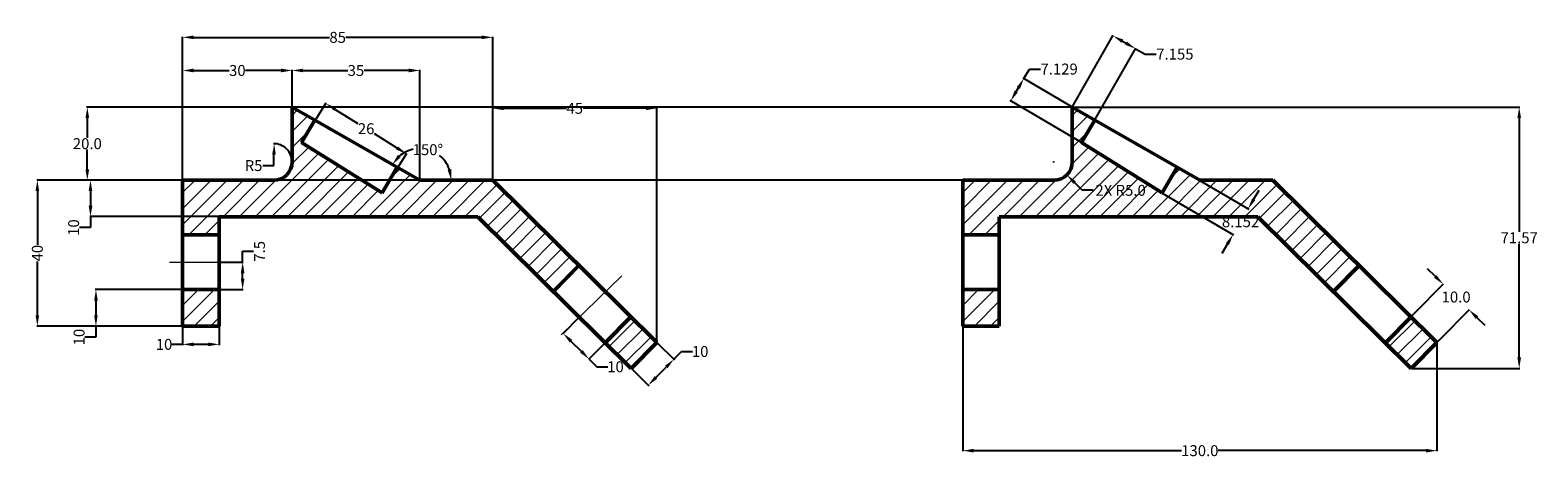
# Model space of a CAD drawing. Units: millimetres. Extents: x 10 to 424, y 8 to 126.
import ezdxf

# ---------------------------------------------------------------- set-up
doc = ezdxf.new("R2010")
doc.units = ezdxf.units.MM
doc.header["$MEASUREMENT"] = 0
doc.linetypes.add('CENTER', pattern=[50.8, 31.75, -6.35, 6.35, -6.35])
for name, color, linetype, lineweight in [('M-CNTR', 4, 'CENTER', 18), ('M-DIMS', 3, 'Continuous', 25), ('M-HATC', 8, 'Continuous', 18), ('M-OUTL', 7, 'Continuous', 50)]:
    doc.layers.add(name, color=color, linetype=linetype, lineweight=lineweight)
doc.styles.get("Standard").update_dxf_attribs({"font": 'arial.ttf'})
doc.dimstyles.get("Standard").update_dxf_attribs({"dimtxt": 3, "dimasz": 3, "dimexe": 0.18, "dimexo": 0.0625, "dimgap": 0.09, "dimtad": 0, "dimtih": 1, "dimtoh": 1, "dimdec": 1, "dimdsep": 46, "dimtxsty": 'Standard', "dimcen": 0.09, "dimadec": 0, "dimazin": 0, "dimtfac": 1, "dimtdec": 1, "dimtofl": 0, "dimtmove": 0, "dimatfit": 3, "dimfxl": 1, "dimtolj": 1, "dimtzin": 0, "dimarcsym": 0})

# ---------------------------------------------------------------- blocks, each defined once
blk = doc.blocks.new('*D1')
at = {"layer": 'Defpoints', "color": 0, "transparency": 16777216}
for p in [(84.8, 94.7), (113.54, 91.62), (106.86, 80.92)]:
    blk.add_point(p, dxfattribs=at)
at = {"layer": 'M-DIMS', "color": 0, "lineweight": -2, "transparency": 16777216}
for p, q in [((84.83, 94.75), (91.58, 105.56)), ((94.03, 103.81), (100.25, 99.93)), ((111, 93.21), (104.78, 97.1)), ((106.89, 80.97), (113.64, 91.77))]:
    blk.add_line(p, q, dxfattribs=at)
at = {"layer": 'M-DIMS', "color": 0, "transparency": 16777216}
for points in [[(94.3, 104.24), (93.77, 103.39), (91.49, 105.4)], [(111.26, 93.63), (110.73, 92.79), (113.54, 91.62)]]:
    blk.add_solid(points, dxfattribs=at)
at = {"layer": 'M-DIMS', "color": 0, "transparency": 16777216, "insert": (102.51, 98.51), "char_height": 3, "attachment_point": 5}
blk.add_mtext('\\A1;26', dxfattribs=at)
blk = doc.blocks.new('*D2')
at = {"layer": 'Defpoints', "color": 0, "transparency": 16777216}
for p in [(137.2, 123.54), (52.2, 84.4), (137.2, 84.4)]:
    blk.add_point(p, dxfattribs=at)
at = {"layer": 'M-DIMS', "color": 0, "lineweight": -2, "transparency": 16777216}
for p, q in [((52.2, 84.46), (52.2, 123.72)), ((55.2, 123.54), (92.44, 123.54)), ((134.2, 123.54), (96.95, 123.54)), ((137.2, 84.46), (137.2, 123.72))]:
    blk.add_line(p, q, dxfattribs=at)
at = {"layer": 'M-DIMS', "color": 0, "transparency": 16777216}
for points in [[(55.2, 124.04), (55.2, 123.04), (52.2, 123.54)], [(134.2, 124.04), (134.2, 123.04), (137.2, 123.54)]]:
    blk.add_solid(points, dxfattribs=at)
at = {"layer": 'M-DIMS', "color": 0, "transparency": 16777216, "insert": (94.7, 123.54), "char_height": 3, "attachment_point": 5}
blk.add_mtext('\\A1;85', dxfattribs=at)
blk = doc.blocks.new('*D3')
at = {"layer": 'Defpoints', "color": 0, "transparency": 16777216}
for p in [(82.2, 114.46), (82.2, 104.4), (52.2, 84.4)]:
    blk.add_point(p, dxfattribs=at)
at = {"layer": 'M-DIMS', "color": 0, "lineweight": -2, "transparency": 16777216}
for p, q in [((52.2, 84.46), (52.2, 114.64)), ((55.2, 114.46), (64.96, 114.46)), ((79.2, 114.46), (69.43, 114.46)), ((82.2, 104.46), (82.2, 114.64))]:
    blk.add_line(p, q, dxfattribs=at)
at = {"layer": 'M-DIMS', "color": 0, "transparency": 16777216}
for points in [[(55.2, 114.96), (55.2, 113.96), (52.2, 114.46)], [(79.2, 114.96), (79.2, 113.96), (82.2, 114.46)]]:
    blk.add_solid(points, dxfattribs=at)
at = {"layer": 'M-DIMS', "color": 0, "transparency": 16777216, "insert": (67.2, 114.46), "char_height": 3, "attachment_point": 5}
blk.add_mtext('\\A1;30', dxfattribs=at)
blk = doc.blocks.new('*D4')
at = {"layer": 'Defpoints', "color": 0, "transparency": 16777216}
for p in [(117.2, 114.46), (82.2, 104.4), (117.2, 84.4)]:
    blk.add_point(p, dxfattribs=at)
at = {"layer": 'M-DIMS', "color": 0, "lineweight": -2, "transparency": 16777216}
for p, q in [((82.2, 104.46), (82.2, 114.64)), ((85.2, 114.46), (97.45, 114.46)), ((114.2, 114.46), (101.94, 114.46)), ((117.2, 84.46), (117.2, 114.64))]:
    blk.add_line(p, q, dxfattribs=at)
at = {"layer": 'M-DIMS', "color": 0, "transparency": 16777216}
for points in [[(85.2, 114.96), (85.2, 113.96), (82.2, 114.46)], [(114.2, 114.96), (114.2, 113.96), (117.2, 114.46)]]:
    blk.add_solid(points, dxfattribs=at)
at = {"layer": 'M-DIMS', "color": 0, "transparency": 16777216, "insert": (99.7, 114.46), "char_height": 3, "attachment_point": 5}
blk.add_mtext('\\A1;35', dxfattribs=at)
blk = doc.blocks.new('*D5')
at = {"layer": 'Defpoints', "color": 0, "transparency": 16777216}
for p in [(77.31, 94.39), (77.2, 89.4)]:
    blk.add_point(p, dxfattribs=at)
at = {"layer": 'M-DIMS', "color": 0, "lineweight": -2, "transparency": 16777216}
for p, q in [((77.17, 88.4), (77.24, 91.4)), ((74.17, 88.4), (77.17, 88.4))]:
    blk.add_line(p, q, dxfattribs=at)
blk.add_arc((77.2, 89.4), 5, 0.7162, 90.7276, dxfattribs=at)
at = {"layer": 'M-DIMS', "color": 0, "transparency": 16777216}
blk.add_solid([(76.74, 91.41), (77.74, 91.38), (77.31, 94.39)], dxfattribs=at)
at = {"layer": 'M-DIMS', "color": 0, "transparency": 16777216, "insert": (71.65, 88.4), "char_height": 3, "attachment_point": 5}
blk.add_mtext('\\A1;R5', dxfattribs=at)
blk = doc.blocks.new('*D6')
at = {"layer": 'Defpoints', "color": 0, "transparency": 16777216}
for p in [(82.2, 104.4), (122.75, 91.04), (117.2, 84.4), (117.2, 84.4), (137.2, 84.4)]:
    blk.add_point(p, dxfattribs=at)
at = {"layer": 'M-DIMS', "color": 0, "lineweight": -2, "transparency": 16777216}
for start, end in [(102.2372, 130.2991), (19.956, 51.1846)]:
    blk.add_arc((117.2, 84.4), 8.66, start, end, dxfattribs=at)
at = {"layer": 'M-DIMS', "color": 0, "transparency": 16777216}
for points in [[(111.98, 90.68), (111.21, 91.32), (109.68, 88.69)], [(125.83, 87.44), (124.84, 87.26), (125.85, 84.4)]]:
    blk.add_solid(points, dxfattribs=at)
at = {"layer": 'M-DIMS', "color": 0, "transparency": 16777216, "insert": (119.42, 92.76), "char_height": 3, "attachment_point": 5}
blk.add_mtext('\\A1;150°', dxfattribs=at)
blk = doc.blocks.new('*D7')
at = {"layer": 'Defpoints', "color": 0, "transparency": 16777216}
for p in [(52.2, 84.4), (26.94, 74.4), (62.2, 74.4)]:
    blk.add_point(p, dxfattribs=at)
at = {"layer": 'M-DIMS', "color": 0, "lineweight": -2, "transparency": 16777216}
for p, q in [((52.13, 84.4), (26.76, 84.4)), ((26.94, 81.4), (26.94, 77.4)), ((26.94, 71.4), (23.94, 71.4)), ((62.13, 74.4), (26.76, 74.4)), ((26.94, 74.4), (26.94, 71.4))]:
    blk.add_line(p, q, dxfattribs=at)
at = {"layer": 'M-DIMS', "color": 0, "transparency": 16777216}
for points in [[(26.44, 81.4), (27.44, 81.4), (26.94, 84.4)], [(26.44, 77.4), (27.44, 77.4), (26.94, 74.4)]]:
    blk.add_solid(points, dxfattribs=at)
at = {"layer": 'M-DIMS', "color": 0, "transparency": 16777216, "insert": (22.32, 71.4), "char_height": 3, "attachment_point": 5, "rotation": 90}
blk.add_mtext('\\A1;10', dxfattribs=at)
blk = doc.blocks.new('*D8')
at = {"layer": 'Defpoints', "color": 0, "transparency": 16777216}
for p in [(52.2, 54.4), (28.43, 44.4), (52.2, 44.4)]:
    blk.add_point(p, dxfattribs=at)
at = {"layer": 'M-DIMS', "color": 0, "lineweight": -2, "transparency": 16777216}
for p, q in [((52.13, 54.4), (28.25, 54.4)), ((28.43, 51.4), (28.43, 47.4)), ((28.43, 41.4), (25.43, 41.4)), ((52.13, 44.4), (28.25, 44.4)), ((28.43, 44.4), (28.43, 41.4))]:
    blk.add_line(p, q, dxfattribs=at)
at = {"layer": 'M-DIMS', "color": 0, "transparency": 16777216}
for points in [[(27.93, 51.4), (28.93, 51.4), (28.43, 54.4)], [(27.93, 47.4), (28.93, 47.4), (28.43, 44.4)]]:
    blk.add_solid(points, dxfattribs=at)
at = {"layer": 'M-DIMS', "color": 0, "transparency": 16777216, "insert": (23.81, 41.4), "char_height": 3, "attachment_point": 5, "rotation": 90}
blk.add_mtext('\\A1;10', dxfattribs=at)
blk = doc.blocks.new('*D9')
at = {"layer": 'Defpoints', "color": 0, "transparency": 16777216}
for p in [(52.2, 44.4), (62.2, 44.4), (52.2, 39.4)]:
    blk.add_point(p, dxfattribs=at)
at = {"layer": 'M-DIMS', "color": 0, "lineweight": -2, "transparency": 16777216}
for p, q in [((52.2, 44.33), (52.2, 39.22)), ((62.2, 44.33), (62.2, 39.22)), ((52.2, 39.4), (49.2, 39.4)), ((59.2, 39.4), (55.2, 39.4))]:
    blk.add_line(p, q, dxfattribs=at)
at = {"layer": 'M-DIMS', "color": 0, "transparency": 16777216}
for points in [[(55.2, 39.9), (55.2, 38.9), (52.2, 39.4)], [(59.2, 39.9), (59.2, 38.9), (62.2, 39.4)]]:
    blk.add_solid(points, dxfattribs=at)
at = {"layer": 'M-DIMS', "color": 0, "transparency": 16777216, "insert": (47.1, 39.4), "char_height": 3, "attachment_point": 5}
blk.add_mtext('\\A1;10', dxfattribs=at)
blk = doc.blocks.new('*D10')
at = {"layer": 'Defpoints', "color": 0, "transparency": 16777216}
for p in [(62.2, 61.9), (68.65, 61.9), (62.2, 54.4)]:
    blk.add_point(p, dxfattribs=at)
at = {"layer": 'M-DIMS', "color": 0, "lineweight": -2, "transparency": 16777216}
for p, q in [((68.65, 61.9), (68.65, 64.9)), ((68.65, 64.9), (71.65, 64.9)), ((62.26, 61.9), (68.83, 61.9)), ((68.65, 57.4), (68.65, 58.9)), ((62.26, 54.4), (68.83, 54.4))]:
    blk.add_line(p, q, dxfattribs=at)
at = {"layer": 'M-DIMS', "color": 0, "transparency": 16777216}
for points in [[(68.15, 58.9), (69.15, 58.9), (68.65, 61.9)], [(68.15, 57.4), (69.15, 57.4), (68.65, 54.4)]]:
    blk.add_solid(points, dxfattribs=at)
at = {"layer": 'M-DIMS', "color": 0, "transparency": 16777216, "insert": (73.27, 64.9), "char_height": 3, "attachment_point": 5, "rotation": 90}
blk.add_mtext('\\A1;7.5', dxfattribs=at)
blk = doc.blocks.new('*D11')
at = {"layer": 'Defpoints', "color": 0, "transparency": 16777216}
for p in [(12.37, 84.4), (52.2, 84.4), (52.2, 44.4)]:
    blk.add_point(p, dxfattribs=at)
at = {"layer": 'M-DIMS', "color": 0, "lineweight": -2, "transparency": 16777216}
for p, q in [((52.13, 84.4), (12.19, 84.4)), ((12.37, 81.4), (12.37, 66.69)), ((12.37, 47.4), (12.37, 62.1)), ((52.13, 44.4), (12.19, 44.4))]:
    blk.add_line(p, q, dxfattribs=at)
at = {"layer": 'M-DIMS', "color": 0, "transparency": 16777216}
for points in [[(11.87, 81.4), (12.87, 81.4), (12.37, 84.4)], [(11.87, 47.4), (12.87, 47.4), (12.37, 44.4)]]:
    blk.add_solid(points, dxfattribs=at)
at = {"layer": 'M-DIMS', "color": 0, "transparency": 16777216, "insert": (12.37, 64.4), "char_height": 3, "attachment_point": 5, "rotation": 90}
blk.add_mtext('\\A1;40', dxfattribs=at)
blk = doc.blocks.new('*D12')
at = {"layer": 'Defpoints', "color": 0, "transparency": 16777216}
for p in [(182.2, 104.09), (137.2, 84.4), (182.2, 39.93)]:
    blk.add_point(p, dxfattribs=at)
at = {"layer": 'M-DIMS', "color": 0, "lineweight": -2, "transparency": 16777216}
for p, q in [((137.2, 84.46), (137.2, 104.27)), ((140.2, 104.09), (157.39, 104.09)), ((179.2, 104.09), (162.01, 104.09)), ((182.2, 40), (182.2, 104.27))]:
    blk.add_line(p, q, dxfattribs=at)
at = {"layer": 'M-DIMS', "color": 0, "transparency": 16777216}
for points in [[(140.2, 104.59), (140.2, 103.59), (137.2, 104.09)], [(179.2, 104.59), (179.2, 103.59), (182.2, 104.09)]]:
    blk.add_solid(points, dxfattribs=at)
at = {"layer": 'M-DIMS', "color": 0, "transparency": 16777216, "insert": (159.7, 104.09), "char_height": 3, "attachment_point": 5}
blk.add_mtext('\\A1;45', dxfattribs=at)
blk = doc.blocks.new('*D13')
at = {"layer": 'Defpoints', "color": 0, "transparency": 16777216}
for p in [(182.2, 39.93), (186.87, 35.32), (175.17, 32.82)]:
    blk.add_point(p, dxfattribs=at)
at = {"layer": 'M-DIMS', "color": 0, "lineweight": -2, "transparency": 16777216}
for p, q in [((182.24, 39.89), (187, 35.19)), ((186.87, 35.32), (188.98, 37.45)), ((188.98, 37.45), (191.98, 37.45)), ((181.95, 30.34), (184.76, 33.18)), ((175.21, 32.78), (179.97, 28.08))]:
    blk.add_line(p, q, dxfattribs=at)
at = {"layer": 'M-DIMS', "color": 0, "transparency": 16777216}
for points in [[(184.41, 33.53), (185.12, 32.83), (186.87, 35.32)], [(181.59, 30.69), (182.31, 29.99), (179.84, 28.2)]]:
    blk.add_solid(points, dxfattribs=at)
at = {"layer": 'M-DIMS', "color": 0, "transparency": 16777216, "insert": (194.07, 37.45), "char_height": 3, "attachment_point": 5}
blk.add_mtext('\\A1;10', dxfattribs=at)
blk = doc.blocks.new('*D14')
at = {"layer": 'Defpoints', "color": 0, "transparency": 16777216}
for p in [(160.95, 46.86), (168.05, 39.85), (163.63, 35.37)]:
    blk.add_point(p, dxfattribs=at)
at = {"layer": 'M-DIMS', "color": 0, "lineweight": -2, "transparency": 16777216}
for p, q in [((160.91, 46.82), (156.4, 42.26)), ((158.66, 40.28), (161.5, 37.48)), ((168.01, 39.81), (163.5, 35.24)), ((163.63, 35.37), (165.76, 33.26)), ((165.76, 33.26), (168.76, 33.26))]:
    blk.add_line(p, q, dxfattribs=at)
at = {"layer": 'M-DIMS', "color": 0, "transparency": 16777216}
for points in [[(159.02, 40.63), (158.31, 39.92), (156.53, 42.39)], [(161.85, 37.84), (161.15, 37.13), (163.63, 35.37)]]:
    blk.add_solid(points, dxfattribs=at)
at = {"layer": 'M-DIMS', "color": 0, "transparency": 16777216, "insert": (170.86, 33.26), "char_height": 3, "attachment_point": 5}
blk.add_mtext('\\A1;10', dxfattribs=at)
blk = doc.blocks.new('BRACKET-SECTION-PROFILE')
for p, q in [((30, 45), (30, 60)), ((65, 40), (30, 60)), ((36.21, 56.45), (32.6, 50.3)), ((54.66, 36.52), (32.6, 50.3)), ((58.79, 43.55), (54.66, 36.52)), ((0, 0), (0, 40)), ((0, 40), (25, 40)), ((65, 40), (85, 40)), ((85, 40), (130, -4.46)), ((10, 0), (10, 30)), ((10, 30), (80.89, 30)), ((80.89, 30), (122.97, -11.57)), ((0, 25), (10, 25)), ((101.63, 9.51), (108.66, 16.62)), ((0, 10), (10, 10)), ((0, 0), (10, 0)), ((115.86, -4.55), (122.89, 2.57)), ((122.97, -11.57), (130, -4.46))]:
    blk.add_line(p, q)
blk.add_arc((25, 45), 5, 270, 0)
blk = doc.blocks.new('*D16')
at = {"layer": 'Defpoints', "color": 0, "transparency": 16777216}
for p in [(266.05, 44.4), (396.05, 39.93), (396.05, 10.27)]:
    blk.add_point(p, dxfattribs=at)
at = {"layer": 'M-DIMS', "color": 0, "lineweight": -2, "transparency": 16777216}
for p, q in [((266.05, 44.33), (266.05, 10.09)), ((396.05, 39.87), (396.05, 10.09)), ((269.05, 10.27), (326.05, 10.27)), ((393.05, 10.27), (336.06, 10.27))]:
    blk.add_line(p, q, dxfattribs=at)
at = {"layer": 'M-DIMS', "color": 0, "transparency": 16777216}
for points in [[(269.05, 10.77), (269.05, 9.77), (266.05, 10.27)], [(393.05, 10.77), (393.05, 9.77), (396.05, 10.27)]]:
    blk.add_solid(points, dxfattribs=at)
at = {"layer": 'M-DIMS', "color": 0, "transparency": 16777216, "insert": (331.05, 10.27), "char_height": 3, "attachment_point": 5}
blk.add_mtext('\\A1;130.0', dxfattribs=at)
blk = doc.blocks.new('*D17')
at = {"layer": 'Defpoints', "color": 0, "transparency": 16777216}
for p in [(296.05, 104.4), (418.6, 104.4), (389.02, 32.82)]:
    blk.add_point(p, dxfattribs=at)
at = {"layer": 'M-DIMS', "color": 0, "lineweight": -2, "transparency": 16777216}
for p, q in [((296.11, 104.4), (418.78, 104.4)), ((418.6, 101.4), (418.6, 70.23)), ((418.6, 35.82), (418.6, 66.99)), ((389.08, 32.82), (418.78, 32.82))]:
    blk.add_line(p, q, dxfattribs=at)
at = {"layer": 'M-DIMS', "color": 0, "transparency": 16777216}
for points in [[(418.1, 101.4), (419.1, 101.4), (418.6, 104.4)], [(418.1, 35.82), (419.1, 35.82), (418.6, 32.82)]]:
    blk.add_solid(points, dxfattribs=at)
at = {"layer": 'M-DIMS', "color": 0, "transparency": 16777216, "insert": (418.6, 68.61), "char_height": 3, "attachment_point": 5}
blk.add_mtext('\\A1;71.57', dxfattribs=at)
blk = doc.blocks.new('*D18')
at = {"layer": 'Defpoints', "color": 0, "transparency": 16777216}
for p in [(26.07, 104.4), (296.05, 104.4), (266.05, 84.4)]:
    blk.add_point(p, dxfattribs=at)
at = {"layer": 'M-DIMS', "color": 0, "lineweight": -2, "transparency": 16777216}
for p, q in [((295.99, 104.4), (25.89, 104.4)), ((26.07, 101.4), (26.07, 96.02)), ((26.07, 87.4), (26.07, 92.77)), ((265.99, 84.4), (25.89, 84.4))]:
    blk.add_line(p, q, dxfattribs=at)
at = {"layer": 'M-DIMS', "color": 0, "transparency": 16777216}
for points in [[(25.57, 101.4), (26.57, 101.4), (26.07, 104.4)], [(25.57, 87.4), (26.57, 87.4), (26.07, 84.4)]]:
    blk.add_solid(points, dxfattribs=at)
at = {"layer": 'M-DIMS', "color": 0, "transparency": 16777216, "insert": (26.07, 94.4), "char_height": 3, "attachment_point": 5}
blk.add_mtext('\\A1;20.0', dxfattribs=at)
blk = doc.blocks.new('*D19')
at = {"layer": 'Defpoints', "color": 0, "transparency": 16777216}
for p in [(313.45, 120.43), (296.05, 104.4), (302.26, 100.85)]:
    blk.add_point(p, dxfattribs=at)
at = {"layer": 'M-DIMS', "color": 0, "lineweight": -2, "transparency": 16777216}
for p, q in [((296.08, 104.45), (307.33, 124.13)), ((302.29, 100.9), (313.54, 120.58)), ((309.84, 122.49), (310.85, 121.91)), ((313.45, 120.43), (316.06, 118.94)), ((316.06, 118.94), (319.06, 118.94))]:
    blk.add_line(p, q, dxfattribs=at)
at = {"layer": 'M-DIMS', "color": 0, "transparency": 16777216}
for points in [[(310.09, 122.92), (309.6, 122.05), (307.24, 123.97)], [(311.09, 122.35), (310.6, 121.48), (313.45, 120.43)]]:
    blk.add_solid(points, dxfattribs=at)
at = {"layer": 'M-DIMS', "color": 0, "transparency": 16777216, "insert": (324.21, 118.94), "char_height": 3, "attachment_point": 5}
blk.add_mtext('\\A1;7.155', dxfattribs=at)
blk = doc.blocks.new('*D20')
at = {"layer": 'Defpoints', "color": 0, "transparency": 16777216}
for p in [(282.82, 112.26), (302.26, 100.85), (298.65, 94.7)]:
    blk.add_point(p, dxfattribs=at)
at = {"layer": 'M-DIMS', "color": 0, "lineweight": -2, "transparency": 16777216}
for p, q in [((302.21, 100.88), (282.66, 112.36)), ((282.82, 112.26), (284.34, 114.85)), ((284.34, 114.85), (287.34, 114.85)), ((280.73, 108.7), (281.3, 109.68)), ((298.6, 94.73), (279.05, 106.21))]:
    blk.add_line(p, q, dxfattribs=at)
at = {"layer": 'M-DIMS', "color": 0, "transparency": 16777216}
for points in [[(280.87, 109.93), (281.73, 109.42), (282.82, 112.26)], [(280.3, 108.96), (281.16, 108.45), (279.21, 106.12)]]:
    blk.add_solid(points, dxfattribs=at)
at = {"layer": 'M-DIMS', "color": 0, "transparency": 16777216, "insert": (292.48, 114.85), "char_height": 3, "attachment_point": 5}
blk.add_mtext('\\A1;7.129', dxfattribs=at)
blk = doc.blocks.new('*D21')
at = {"layer": 'Defpoints', "color": 0, "transparency": 16777216}
for p in [(324.84, 87.95), (320.71, 80.92), (340.16, 69.5)]:
    blk.add_point(p, dxfattribs=at)
at = {"layer": 'M-DIMS', "color": 0, "lineweight": -2, "transparency": 16777216}
for p, q in [((324.89, 87.91), (344.44, 76.44)), ((320.76, 80.88), (340.31, 69.41)), ((345.8, 79.11), (347.32, 81.7)), ((338.64, 66.91), (337.12, 64.32))]:
    blk.add_line(p, q, dxfattribs=at)
at = {"layer": 'M-DIMS', "color": 0, "transparency": 16777216}
for points in [[(345.37, 79.37), (346.23, 78.86), (344.28, 76.53)], [(338.21, 67.16), (339.07, 66.66), (340.16, 69.5)]]:
    blk.add_solid(points, dxfattribs=at)
at = {"layer": 'M-DIMS', "color": 0, "transparency": 16777216, "insert": (342.22, 73.01), "char_height": 3, "attachment_point": 5}
blk.add_mtext('\\A1;8.152', dxfattribs=at)
blk = doc.blocks.new('*D22')
at = {"layer": 'Defpoints', "color": 0, "transparency": 16777216}
for p in [(404.87, 48.86), (381.91, 39.85), (389.02, 32.82)]:
    blk.add_point(p, dxfattribs=at)
at = {"layer": 'M-DIMS', "color": 0, "lineweight": -2, "transparency": 16777216}
for p, q in [((395.62, 58), (393.49, 60.11)), ((381.95, 39.89), (397.88, 56.02)), ((389.07, 32.87), (405, 48.99)), ((407.01, 46.75), (409.14, 44.65))]:
    blk.add_line(p, q, dxfattribs=at)
at = {"layer": 'M-DIMS', "color": 0, "transparency": 16777216}
for points in [[(395.98, 58.35), (395.27, 57.64), (397.76, 55.89)], [(407.36, 47.11), (406.65, 46.4), (404.87, 48.86)]]:
    blk.add_solid(points, dxfattribs=at)
at = {"layer": 'M-DIMS', "color": 0, "transparency": 16777216, "insert": (401.31, 52.38), "char_height": 3, "attachment_point": 5}
blk.add_mtext('\\A1;10.0', dxfattribs=at)
blk = doc.blocks.new('*D23')
at = {"layer": 'Defpoints', "color": 0, "transparency": 16777216}
for p in [(291.05, 89.4), (294.59, 85.86)]:
    blk.add_point(p, dxfattribs=at)
at = {"layer": 'M-DIMS', "color": 0, "lineweight": -2, "transparency": 16777216}
for p, q in [((290.96, 89.4), (291.14, 89.4)), ((291.05, 89.31), (291.05, 89.49)), ((298.83, 81.62), (296.71, 83.74)), ((301.83, 81.62), (298.83, 81.62))]:
    blk.add_line(p, q, dxfattribs=at)
at = {"layer": 'M-DIMS', "color": 0, "transparency": 16777216}
blk.add_solid([(297.06, 84.09), (296.35, 83.39), (294.59, 85.86)], dxfattribs=at)
at = {"layer": 'M-DIMS', "color": 0, "transparency": 16777216, "insert": (309.33, 81.62), "char_height": 3, "attachment_point": 5}
blk.add_mtext('\\A1;2X R5.0', dxfattribs=at)

msp = doc.modelspace()

# ---------------------------------------------------------------- hatches: boundary and pattern name
at = {"layer": 'M-HATC'}
h = msp.add_hatch(dxfattribs=at)
h.set_pattern_fill('ANSI31', color=256, scale=25)
h.set_pattern_definition([(45, (37.2045, 39.4764), (-2.20971, 2.20971), [])])
h.paths.add_polyline_path([(182.1956, 39.9348), (175.0821, 46.9632), (168.0538, 39.8497), (175.1673, 32.8213)])
h.paths.add_polyline_path([(137.1956, 84.3961), (117.1956, 84.3961), (110.9836, 87.9458), (106.8557, 80.9163), (84.798, 94.6992), (88.4077, 100.8463), (82.1956, 104.3961), (82.1956, 89.3961, -0.41421356), (77.1956, 84.3961), (52.1956, 84.3961), (52.1956, 69.3961), (62.1956, 69.3961), (62.1956, 74.3961), (133.0887, 74.3961), (153.8267, 53.9064), (160.8551, 61.0199)])
h.paths.add_polyline_path([(52.1956, 44.3961), (62.1956, 44.3961), (62.1956, 54.3961), (52.1956, 54.3961)])
h = msp.add_hatch(dxfattribs=at)
h.set_pattern_fill('ANSI31', color=256, scale=25)
h.set_pattern_definition([(45, (251.0596, 39.4764), (-2.20971, 2.20971), [])])
h.paths.add_polyline_path([(396.0507, 39.9348), (388.9372, 46.9632), (381.9088, 39.8497), (389.0223, 32.8213)])
h.paths.add_polyline_path([(351.0507, 84.3961), (331.0507, 84.3961), (324.8386, 87.9458), (320.7108, 80.9163), (298.6531, 94.6992), (302.2627, 100.8463), (296.0507, 104.3961), (296.0507, 89.3961, -0.41421356), (291.0507, 84.3961), (266.0507, 84.3961), (266.0507, 69.3961), (276.0507, 69.3961), (276.0507, 74.3961), (346.9438, 74.3961), (367.6818, 53.9064), (374.7101, 61.0199)])
h.paths.add_polyline_path([(266.0507, 44.3961), (276.0507, 44.3961), (276.0507, 54.3961), (266.0507, 54.3961)])

# ---------------------------------------------------------------- linework, layer by layer
at = {"layer": 'M-CNTR'}
for p, q in [((48.6225, 61.8961), (65.8125, 61.8961)), ((155.9806, 42.0295), (172.5991, 58.1859))]:
    msp.add_line(p, q, dxfattribs=at)

# ---------------------------------------------------------------- block references
at = {"layer": 'M-OUTL'}
for p in [(52.1956, 44.3961), (266.0507, 44.3961)]:
    msp.add_blockref('BRACKET-SECTION-PROFILE', p, dxfattribs=at)

# ---------------------------------------------------------------- dimensions: what is measured, and where the dimension line sits
at = {"layer": 'M-DIMS', "transparency": 33554610}
for base, p1, p2, picture, middle in [((137.1956, 123.5399), (52.1956, 84.3961), (137.1956, 84.3961), '*D2', (94.6956, 123.5399)), ((82.1956, 114.4587), (52.1956, 84.3961), (82.1956, 104.3961), '*D3', (67.1956, 114.4587)), ((117.1956, 114.4587), (82.1956, 104.3961), (117.1956, 84.3961), '*D4', (99.6956, 114.4587)), ((182.1956, 104.0892), (137.1956, 84.3961), (182.1956, 39.9348), '*D12', (159.6956, 104.0892)), ((52.1956, 39.4014), (62.1956, 44.3961), (52.1956, 44.3961), '*D9', (47.1032, 39.4014))]:
    dim = msp.add_linear_dim(base=base, p1=p1, p2=p2, dimstyle='Standard', override={"dimclrd": 0, "dimclre": 0, "dimclrt": 0}, dxfattribs=at)
    dim.commit()
    dim.dimension.update_dxf_attribs({"geometry": picture, "text_midpoint": middle})
at = {"layer": 'M-DIMS'}
for base, p1, p2, angle, override, picture, middle in [((313.4507, 120.4252), (296.0507, 104.3961), (302.2627, 100.8463), 330.255119, {"dimdec": 3, "dimlfac": 1, "dimrnd": 0, "dimzin": 0, "dimdsep": 46, "dimlunit": 2}, '*D19', (324.2061, 118.9368)), ((282.8175, 112.265), (298.6531, 94.6992), (302.2627, 100.8463), 59.577661, {"dimdec": 3, "dimlfac": 1, "dimrnd": 0, "dimzin": 0, "dimdsep": 46, "dimlunit": 2}, '*D20', (292.4792, 114.8519)), ((26.0725, 104.3961), (266.0507, 84.3961), (296.0507, 104.3961), 90, {"dimdec": 1, "dimlfac": 1, "dimrnd": 0, "dimzin": 0, "dimdsep": 46, "dimlunit": 2}, '*D18', (26.0725, 94.3961)), ((418.6007, 104.3961), (389.0223, 32.8213), (296.0507, 104.3961), 90, {"dimdec": 2, "dimlfac": 1, "dimrnd": 0, "dimzin": 0, "dimdsep": 46, "dimlunit": 2}, '*D17', (418.6007, 68.6087)), ((340.156, 69.4977), (324.8386, 87.9458), (320.7108, 80.9163), 239.577661, {"dimdec": 3, "dimlfac": 1, "dimrnd": 0, "dimzin": 0, "dimdsep": 46, "dimlunit": 2}, '*D21', (342.22, 73.0124)), ((404.8713, 48.8623), (381.9088, 39.8497), (389.0223, 32.8213), 315.345072, {"dimdec": 1, "dimlfac": 1, "dimrnd": 0, "dimzin": 0, "dimdsep": 46, "dimlunit": 2}, '*D22', (401.3145, 52.3765))]:
    dim = msp.add_linear_dim(base=base, p1=p1, p2=p2, angle=angle, dimstyle='Standard', override=override, dxfattribs=at)
    dim.commit()
    dim.dimension.update_dxf_attribs({"geometry": picture, "text_midpoint": middle})
at = {"layer": 'M-DIMS', "transparency": 33554610}
dim = msp.add_angular_dim_2l(base=(122.7504, 91.036), line1=((117.1956, 84.3961), (82.1956, 104.3961)), line2=((117.1956, 84.3961), (137.1956, 84.3961)), dimstyle='Standard', override={"dimclrd": 0, "dimclre": 0, "dimclrt": 0}, dxfattribs=at)
dim.commit()
dim.dimension.update_dxf_attribs({"geometry": '*D6', "text_midpoint": (119.4176, 92.7631)})
for p1, p2, distance, picture, middle in [((84.798, 94.6992), (106.8557, 80.9163), 12.6211, '*D1', (102.5149, 98.5112)), ((160.9539, 46.8645), (168.0538, 39.8497), -6.2932, '*D14', (170.8571, 33.2645)), ((175.1673, 32.8213), (182.1956, 39.9348), -6.5717, '*D13', (194.0713, 37.4501))]:
    dim = msp.add_aligned_dim(p1=p1, p2=p2, distance=distance, dimstyle='Standard', override={"dimclrd": 0, "dimclre": 0, "dimclrt": 0}, dxfattribs=at)
    dim.commit()
    dim.dimension.update_dxf_attribs({"geometry": picture, "text_midpoint": middle})
dim = msp.add_radius_dim(center=(77.1956, 89.3961), mpoint=(77.3121, 94.3947), dimstyle='Standard', override={"dimclrd": 0, "dimclre": 0, "dimclrt": 0}, dxfattribs=at)
dim.commit()
dim.dimension.update_dxf_attribs({"geometry": '*D5', "text_midpoint": (71.6522, 88.3963), "dimtype": 164})
at = {"layer": 'M-DIMS'}
dim = msp.add_radius_dim(center=(291.0507, 89.3961), mpoint=(294.5864, 85.8606), text='2X <>', dimstyle='Standard', override={"dimdec": 1, "dimlfac": 1, "dimrnd": 0, "dimzin": 0, "dimdsep": 46, "dimlunit": 2}, dxfattribs=at)
dim.commit()
dim.dimension.update_dxf_attribs({"geometry": '*D23', "text_midpoint": (309.3291, 81.6182)})
at = {"layer": 'M-DIMS', "transparency": 33554610}
for base, p1, p2, picture, middle in [((12.3684, 84.3961), (52.1956, 44.3961), (52.1956, 84.3961), '*D11', (12.3684, 64.3961)), ((26.9421, 74.3961), (52.1956, 84.3961), (62.1956, 74.3961), '*D7', (22.3204, 71.3961)), ((68.6497, 61.8961), (62.1956, 54.3961), (62.1956, 61.8961), '*D10', (73.2653, 64.8961)), ((28.432, 44.3961), (52.1956, 54.3961), (52.1956, 44.3961), '*D8', (23.8103, 41.3961))]:
    dim = msp.add_linear_dim(base=base, p1=p1, p2=p2, angle=90, dimstyle='Standard', override={"dimclrd": 0, "dimclre": 0, "dimclrt": 0}, dxfattribs=at)
    dim.commit()
    dim.dimension.update_dxf_attribs({"geometry": picture, "text_midpoint": middle, "text_rotation": 90})
at = {"layer": 'M-DIMS'}
dim = msp.add_linear_dim(base=(396.0507, 10.2713), p1=(266.0507, 44.3961), p2=(396.0507, 39.9348), dimstyle='Standard', override={"dimdec": 1, "dimlfac": 1, "dimrnd": 0, "dimzin": 0, "dimdsep": 46, "dimlunit": 2}, dxfattribs=at)
dim.commit()
dim.dimension.update_dxf_attribs({"geometry": '*D16', "text_midpoint": (331.0507, 10.2713)})

doc.saveas('drawing.dxf')
